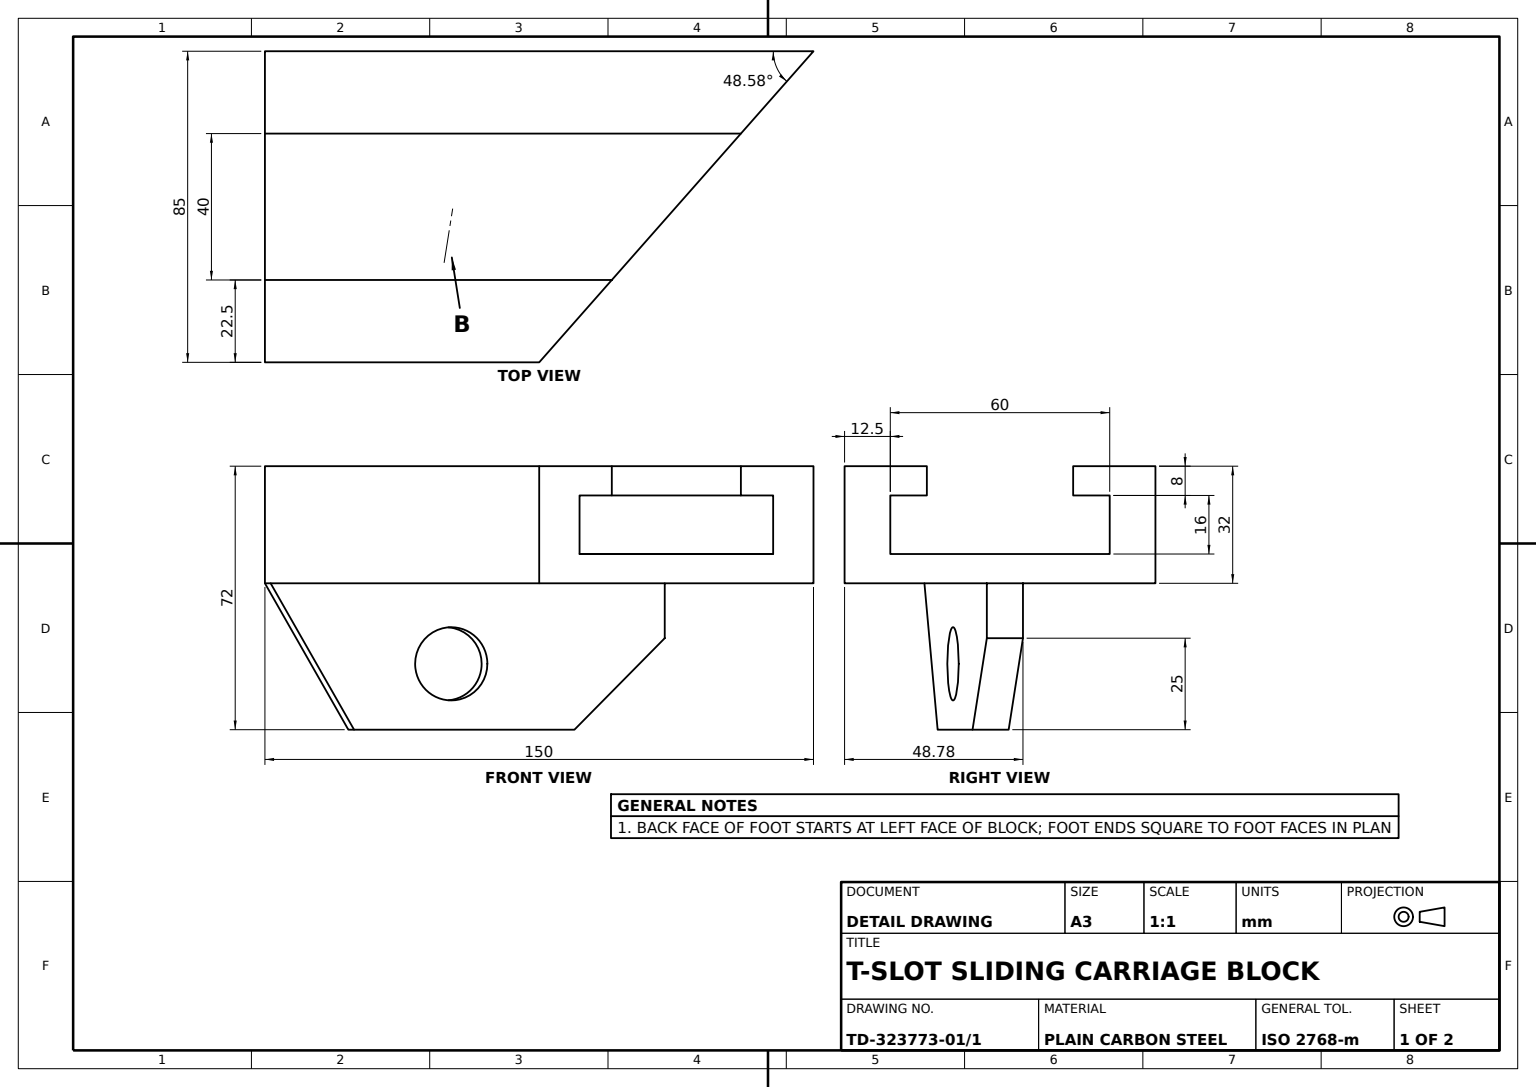
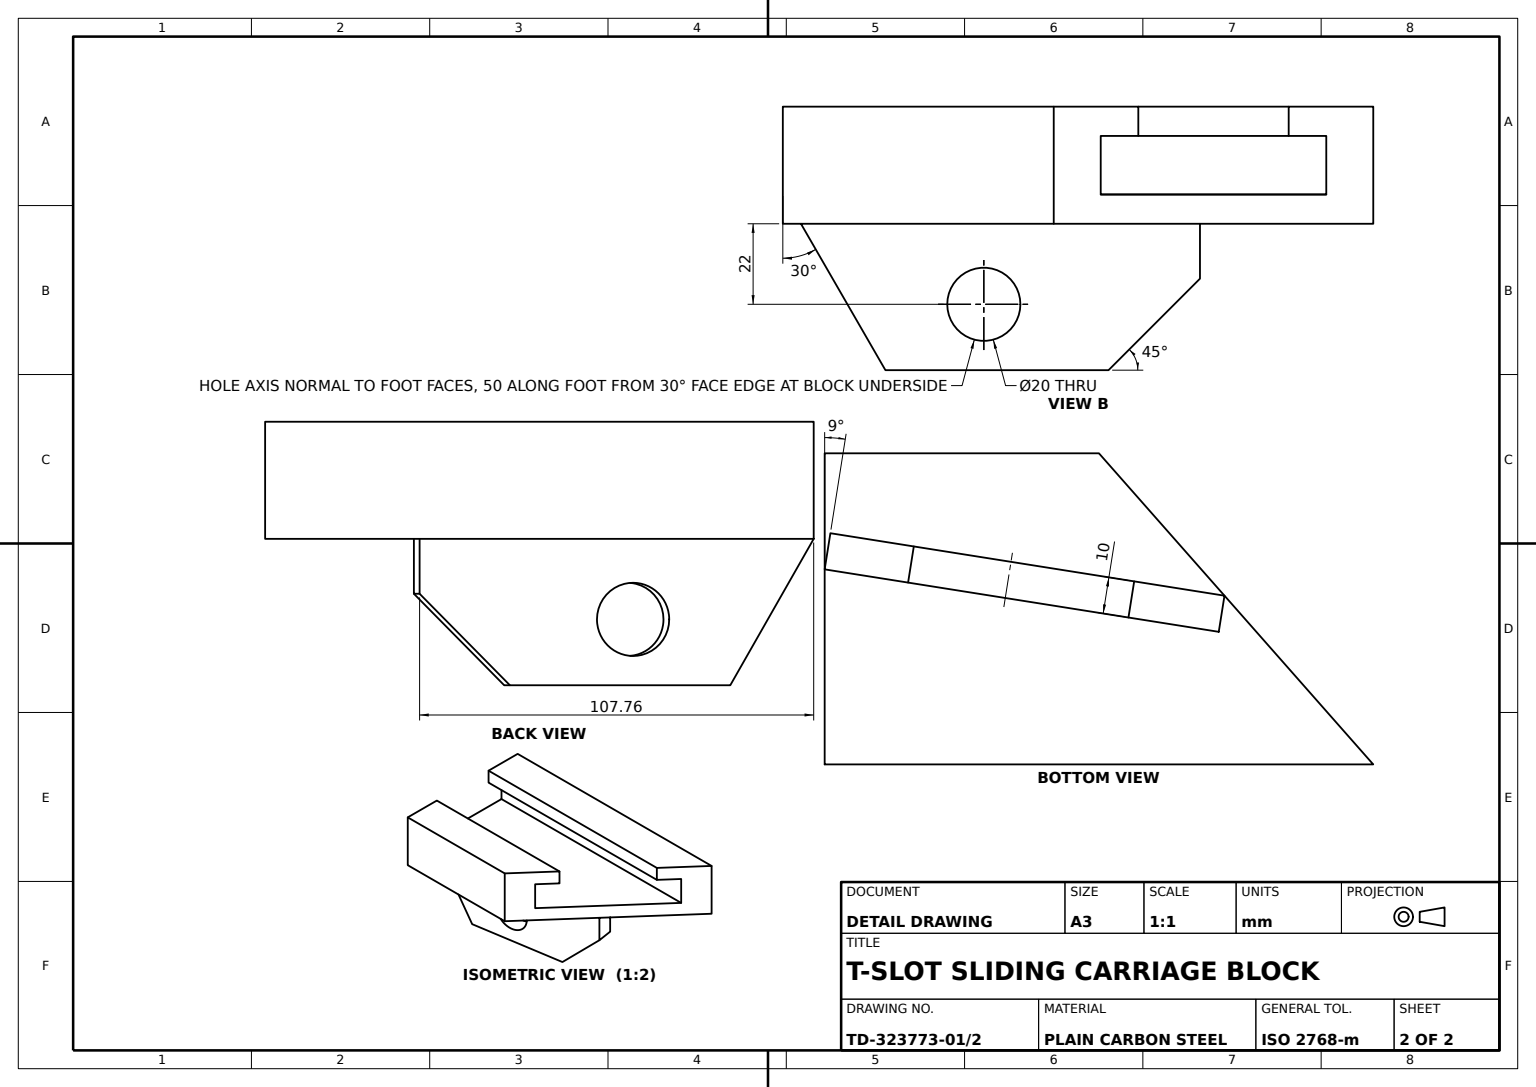
from build123d import *

# Parameters (mm, degrees)
BASE_BLOCK_150X85X32_DEPTH = 32
T_SLOT_CUT_DEPTH           = 160.154798859
T_SLOT_CUT_DEPTH_BACK      = 160.154798859
TAPERED_FOOT_BOSS_DEPTH    = 40
FOOT_RELIEF_CUT_DEPTH      = 101.347613869
FOOT_RELIEF_CUT_DEPTH_BACK = 101.347613869
FOOT_RELIEF_SKETCH_R       = 10


with BuildPart() as part:
    # Base Block Sketch → Base Block 150x85x32 (new body)
    with BuildSketch(Plane(origin=(0, 0, 0), x_dir=(1, 0, 0), z_dir=(0, 1, 0))):
        Polygon((-75, 42.5), (75, 42.5), (0, -42.5), (-75, -42.5), align=None)
    extrude(amount=BASE_BLOCK_150X85X32_DEPTH)

    # T-Slot Sketch → T-Slot Cut (cut, two sides: drawn at the far end of the back side and taken through both)
    with BuildSketch(Plane.ZY.offset(75).offset(-T_SLOT_CUT_DEPTH_BACK)):
        Polygon((-20, 32), (-20, 24), (-30, 24), (-30, 8), (30, 8), (30, 24), (20, 24), (20, 32), align=None)
    extrude(amount=T_SLOT_CUT_DEPTH + T_SLOT_CUT_DEPTH_BACK, mode=Mode.SUBTRACT)

    # Tapered Foot Sketch → Tapered Foot Boss (add)
    with BuildSketch(Plane.XZ):
        Polygon((-75, 10.790645392), (-73.43565535, 20.667528798), (34.323374911, 3.6001751), (32.759030261, -6.276708306), align=None)
    extrude(amount=TAPERED_FOOT_BOSS_DEPTH)

    # Foot Relief Sketch → Foot Relief Cut (cut, two sides: drawn at the far end of the back side and taken through both)
    with BuildSketch(Plane(origin=(1.396210415, 0, 8.815325621), x_dir=(0.9876883405951378, 0, -0.15643446504023126), z_dir=(0.15643446504023126, 0, 0.9876883405951378)).offset(-FOOT_RELIEF_CUT_DEPTH_BACK)):
        Polygon((33.337605744, -15), (8.337605744, -40), (33.337605744, -40), align=None)
        with Locations((-25.764654384, -22)):
            Circle(FOOT_RELIEF_SKETCH_R)
        Polygon((-52.670643616, -40), (-75.764654384, 0), (-75.764654384, -40), align=None)
    extrude(amount=FOOT_RELIEF_CUT_DEPTH + FOOT_RELIEF_CUT_DEPTH_BACK, mode=Mode.SUBTRACT)


solid = part.part
